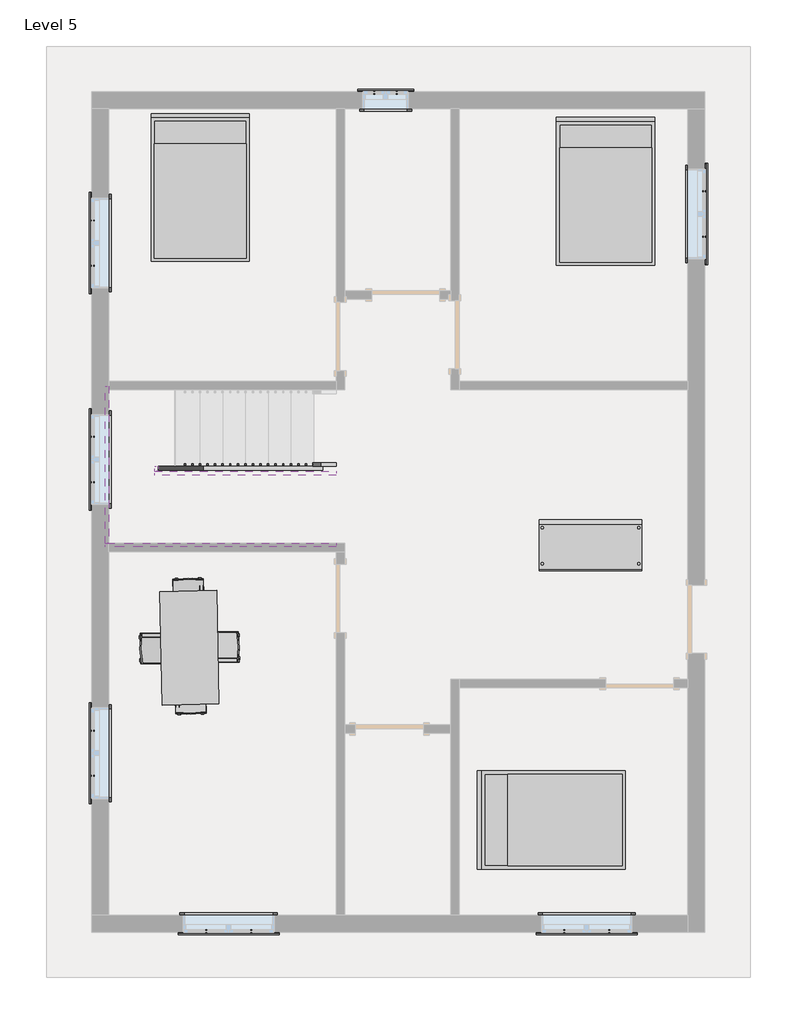
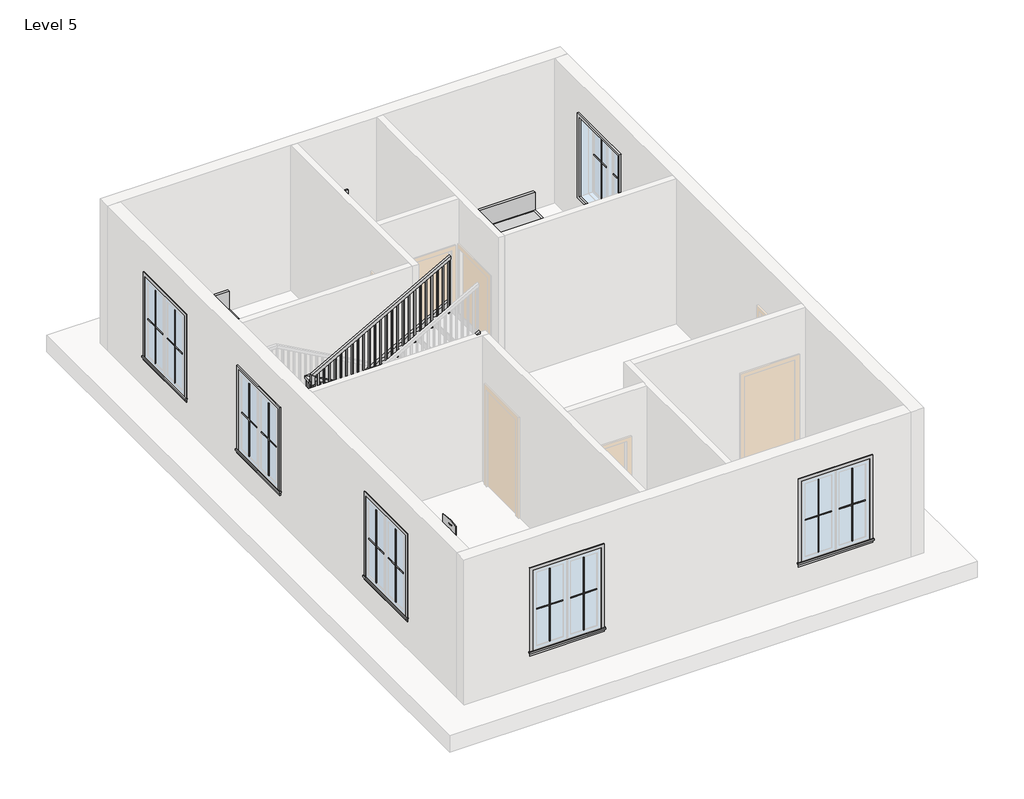
# One storey, part 2 of 2: 29 proxies, 6 members, 4 furniture elements, 1 railing.
"""IFC4 building model written with IfcOpenShell, lengths in millimetres."""

from ifc_helpers import new_model, si_unit, frame, origin, place, context, project, spatial, polyline, outline, extrude, faceted_brep, transform, mapped, element, save
from components import modern_coffee_table_17989_modern_coffee_table_17989_d3a860c8, muntin_pattern_2x2_muntin_pattern_2x2_6dad3731, muntin_pattern_2x2_muntin_pattern_2x2_a30a3345, muntin_pattern_2x2_muntin_pattern_2x2_53152e2c, muntin_pattern_2x2_muntin_pattern_2x2_e8f3e573, trim_window_exterior_flat_with_sill_92b9b949, trim_window_exterior_flat_with_sill_a665a915, trim_window_interior_flat_picture_frame_3bb882cf, trim_window_interior_flat_picture_frame_d485c387, bed_17739_bed_17739_15c61121, dining_table_w_chairs_11374_0cdfc61b

model = new_model("IFC4")

# Units and contexts
model_context = context("Model", 3, world=origin())
ifc_project = project(units=[si_unit("LENGTHUNIT", "METRE", prefix="MILLI")], contexts=[model_context])

# Site, building, storey
site = spatial("IfcSite", under=ifc_project)
building = spatial("IfcBuilding", under=site)
storey = spatial("IfcBuildingStorey", under=building, Name="Level 5", Elevation=12192.0)

# Proxies
placement = place(None, origin())
modern_coffee_table_17989_modern_coffee_table_17989_shape = modern_coffee_table_17989_modern_coffee_table_17989_d3a860c8(model_context)
element("IfcBuildingElementProxy", 1, Name="Modern_Coffee_Table_17989 : Modern_Coffee_Table_17989", ObjectType="Modern_Coffee_Table_17989 : Modern_Coffee_Table_17989", at=placement, inside=storey, context=model_context, shape_type="MappedRepresentation", body=[
    mapped(modern_coffee_table_17989_modern_coffee_table_17989_shape, transform((7937.5, 8234.1992646, 12192.0), x_axis=(1.0, 0.0, 0.0), y_axis=(0.0, 1.0, 0.0), z_axis=(0.0, 0.0, 1.0))),
])
muntin_pattern_2x2_muntin_pattern_2x2_shape = muntin_pattern_2x2_muntin_pattern_2x2_6dad3731(model_context)
element("IfcBuildingElementProxy", 2, Name="Muntin Pattern_2x2 : Muntin Pattern_2x2", ObjectType="Muntin Pattern_2x2 : Muntin Pattern_2x2", at=placement, inside=storey, context=model_context, shape_type="MappedRepresentation", body=[
    mapped(muntin_pattern_2x2_muntin_pattern_2x2_shape, transform((7961.3125, 2701.925, 13176.25), x_axis=(-1.0, 0.0, 0.0), y_axis=(0.0, -1.0, 0.0), z_axis=(0.0, 0.0, 1.0))),
])
element("IfcBuildingElementProxy", 3, Name="Muntin Pattern_2x2 : Muntin Pattern_2x2", ObjectType="Muntin Pattern_2x2 : Muntin Pattern_2x2", at=placement, inside=storey, context=model_context, shape_type="MappedRepresentation", body=[
    mapped(muntin_pattern_2x2_muntin_pattern_2x2_shape, transform((3154.3625, 2701.925, 13176.25), x_axis=(-1.0, 0.0, 0.0), y_axis=(0.0, -1.0, 0.0), z_axis=(0.0, 0.0, 1.0))),
])
element("IfcBuildingElementProxy", 4, Name="Muntin Pattern_2x2 : Muntin Pattern_2x2", ObjectType="Muntin Pattern_2x2 : Muntin Pattern_2x2", at=placement, inside=storey, context=model_context, shape_type="MappedRepresentation", body=[
    mapped(muntin_pattern_2x2_muntin_pattern_2x2_shape, transform((1025.525, 4789.4875, 13176.25), x_axis=(0.0, 1.0, 0.0), y_axis=(-1.0, 0.0, 0.0), z_axis=(0.0, 0.0, 1.0))),
])
element("IfcBuildingElementProxy", 5, Name="Muntin Pattern_2x2 : Muntin Pattern_2x2", ObjectType="Muntin Pattern_2x2 : Muntin Pattern_2x2", at=placement, inside=storey, context=model_context, shape_type="MappedRepresentation", body=[
    mapped(muntin_pattern_2x2_muntin_pattern_2x2_shape, transform((1025.525, 8732.8375, 13176.25), x_axis=(0.0, 1.0, 0.0), y_axis=(-1.0, 0.0, 0.0), z_axis=(0.0, 0.0, 1.0))),
])
element("IfcBuildingElementProxy", 6, Name="Muntin Pattern_2x2 : Muntin Pattern_2x2", ObjectType="Muntin Pattern_2x2 : Muntin Pattern_2x2", at=placement, inside=storey, context=model_context, shape_type="MappedRepresentation", body=[
    mapped(muntin_pattern_2x2_muntin_pattern_2x2_shape, transform((1025.525, 11637.9625, 13176.25), x_axis=(0.0, 1.0, 0.0), y_axis=(-1.0, 0.0, 0.0), z_axis=(0.0, 0.0, 1.0))),
])
element("IfcBuildingElementProxy", 7, Name="Muntin Pattern_2x2 : Muntin Pattern_2x2", ObjectType="Muntin Pattern_2x2 : Muntin Pattern_2x2", at=placement, inside=storey, context=model_context, shape_type="MappedRepresentation", body=[
    mapped(muntin_pattern_2x2_muntin_pattern_2x2_shape, transform((9236.075, 12634.9125, 13176.25), x_axis=(0.0, -1.0, 0.0), y_axis=(1.0, 0.0, 0.0), z_axis=(0.0, 0.0, 1.0))),
])
muntin_pattern_2x2_muntin_pattern_2x2_2_shape = muntin_pattern_2x2_muntin_pattern_2x2_a30a3345(model_context)
element("IfcBuildingElementProxy", 8, Name="Muntin Pattern_2x2 : Muntin Pattern_2x2", ObjectType="Muntin Pattern_2x2 : Muntin Pattern_2x2", at=placement, inside=storey, context=model_context, shape_type="MappedRepresentation", body=[
    mapped(muntin_pattern_2x2_muntin_pattern_2x2_2_shape, transform((7354.8875, 2701.925, 13176.25), x_axis=(1.0, 0.0, 0.0), y_axis=(0.0, 1.0, 0.0), z_axis=(0.0, 0.0, 1.0))),
])
element("IfcBuildingElementProxy", 9, Name="Muntin Pattern_2x2 : Muntin Pattern_2x2", ObjectType="Muntin Pattern_2x2 : Muntin Pattern_2x2", at=placement, inside=storey, context=model_context, shape_type="MappedRepresentation", body=[
    mapped(muntin_pattern_2x2_muntin_pattern_2x2_2_shape, transform((2547.9375, 2701.925, 13176.25), x_axis=(1.0, 0.0, 0.0), y_axis=(0.0, 1.0, 0.0), z_axis=(0.0, 0.0, 1.0))),
])
element("IfcBuildingElementProxy", 10, Name="Muntin Pattern_2x2 : Muntin Pattern_2x2", ObjectType="Muntin Pattern_2x2 : Muntin Pattern_2x2", at=placement, inside=storey, context=model_context, shape_type="MappedRepresentation", body=[
    mapped(muntin_pattern_2x2_muntin_pattern_2x2_2_shape, transform((1025.525, 5395.9125, 13176.25), x_axis=(0.0, -1.0, 0.0), y_axis=(1.0, 0.0, 0.0), z_axis=(0.0, 0.0, 1.0))),
])
element("IfcBuildingElementProxy", 11, Name="Muntin Pattern_2x2 : Muntin Pattern_2x2", ObjectType="Muntin Pattern_2x2 : Muntin Pattern_2x2", at=placement, inside=storey, context=model_context, shape_type="MappedRepresentation", body=[
    mapped(muntin_pattern_2x2_muntin_pattern_2x2_2_shape, transform((1025.525, 9339.2625, 13176.25), x_axis=(0.0, -1.0, 0.0), y_axis=(1.0, 0.0, 0.0), z_axis=(0.0, 0.0, 1.0))),
])
element("IfcBuildingElementProxy", 12, Name="Muntin Pattern_2x2 : Muntin Pattern_2x2", ObjectType="Muntin Pattern_2x2 : Muntin Pattern_2x2", at=placement, inside=storey, context=model_context, shape_type="MappedRepresentation", body=[
    mapped(muntin_pattern_2x2_muntin_pattern_2x2_2_shape, transform((1025.525, 12244.3875, 13176.25), x_axis=(0.0, -1.0, 0.0), y_axis=(1.0, 0.0, 0.0), z_axis=(0.0, 0.0, 1.0))),
])
element("IfcBuildingElementProxy", 13, Name="Muntin Pattern_2x2 : Muntin Pattern_2x2", ObjectType="Muntin Pattern_2x2 : Muntin Pattern_2x2", at=placement, inside=storey, context=model_context, shape_type="MappedRepresentation", body=[
    mapped(muntin_pattern_2x2_muntin_pattern_2x2_2_shape, transform((9236.075, 12028.4875, 13176.25), x_axis=(0.0, 1.0, 0.0), y_axis=(-1.0, 0.0, 0.0), z_axis=(0.0, 0.0, 1.0))),
])
muntin_pattern_2x2_muntin_pattern_2x2_3_shape = muntin_pattern_2x2_muntin_pattern_2x2_53152e2c(model_context)
element("IfcBuildingElementProxy", 14, Name="Muntin Pattern_2x2 : Muntin Pattern_2x2", ObjectType="Muntin Pattern_2x2 : Muntin Pattern_2x2", at=placement, inside=storey, context=model_context, shape_type="MappedRepresentation", body=[
    mapped(muntin_pattern_2x2_muntin_pattern_2x2_3_shape, transform((4808.5375, 13960.475, 13176.25), x_axis=(1.0, 0.0, 0.0), y_axis=(0.0, 1.0, 0.0), z_axis=(0.0, 0.0, 1.0))),
])
muntin_pattern_2x2_muntin_pattern_2x2_4_shape = muntin_pattern_2x2_muntin_pattern_2x2_e8f3e573(model_context)
element("IfcBuildingElementProxy", 15, Name="Muntin Pattern_2x2 : Muntin Pattern_2x2", ObjectType="Muntin Pattern_2x2 : Muntin Pattern_2x2", at=placement, inside=storey, context=model_context, shape_type="MappedRepresentation", body=[
    mapped(muntin_pattern_2x2_muntin_pattern_2x2_4_shape, transform((5110.1625, 13960.475, 13176.25), x_axis=(-1.0, 0.0, 0.0), y_axis=(0.0, -1.0, 0.0), z_axis=(0.0, 0.0, 1.0))),
])
trim_window_exterior_flat_with_sill_shape = trim_window_exterior_flat_with_sill_92b9b949(model_context)
element("IfcBuildingElementProxy", 16, Name="Trim-Window-Exterior-Flat : with Sill", ObjectType="Trim-Window-Exterior-Flat : with Sill", at=placement, inside=storey, context=model_context, shape_type="MappedRepresentation", body=[
    mapped(trim_window_exterior_flat_with_sill_shape, transform((7658.1, 2692.4, 14630.4), x_axis=(1.0, 0.0, 0.0), y_axis=(0.0, 0.0, 1.0), z_axis=(0.0, -1.0, 0.0))),
])
element("IfcBuildingElementProxy", 17, Name="Trim-Window-Exterior-Flat : with Sill", ObjectType="Trim-Window-Exterior-Flat : with Sill", at=placement, inside=storey, context=model_context, shape_type="MappedRepresentation", body=[
    mapped(trim_window_exterior_flat_with_sill_shape, transform((2851.15, 2692.4, 14630.4), x_axis=(1.0, 0.0, 0.0), y_axis=(0.0, 0.0, 1.0), z_axis=(0.0, -1.0, 0.0))),
])
element("IfcBuildingElementProxy", 18, Name="Trim-Window-Exterior-Flat : with Sill", ObjectType="Trim-Window-Exterior-Flat : with Sill", at=placement, inside=storey, context=model_context, shape_type="MappedRepresentation", body=[
    mapped(trim_window_exterior_flat_with_sill_shape, transform((1016.0, 5092.7, 14630.4), x_axis=(0.0, -1.0, 0.0), y_axis=(0.0, 0.0, 1.0), z_axis=(-1.0, 0.0, 0.0))),
])
element("IfcBuildingElementProxy", 19, Name="Trim-Window-Exterior-Flat : with Sill", ObjectType="Trim-Window-Exterior-Flat : with Sill", at=placement, inside=storey, context=model_context, shape_type="MappedRepresentation", body=[
    mapped(trim_window_exterior_flat_with_sill_shape, transform((1016.0, 9036.05, 14630.4), x_axis=(0.0, -1.0, 0.0), y_axis=(0.0, 0.0, 1.0), z_axis=(-1.0, 0.0, 0.0))),
])
element("IfcBuildingElementProxy", 20, Name="Trim-Window-Exterior-Flat : with Sill", ObjectType="Trim-Window-Exterior-Flat : with Sill", at=placement, inside=storey, context=model_context, shape_type="MappedRepresentation", body=[
    mapped(trim_window_exterior_flat_with_sill_shape, transform((1016.0, 11941.175, 14630.4), x_axis=(0.0, -1.0, 0.0), y_axis=(0.0, 0.0, 1.0), z_axis=(-1.0, 0.0, 0.0))),
])
element("IfcBuildingElementProxy", 21, Name="Trim-Window-Exterior-Flat : with Sill", ObjectType="Trim-Window-Exterior-Flat : with Sill", at=placement, inside=storey, context=model_context, shape_type="MappedRepresentation", body=[
    mapped(trim_window_exterior_flat_with_sill_shape, transform((9245.6, 12331.7, 14630.4), x_axis=(0.0, 1.0, 0.0), y_axis=(0.0, 0.0, 1.0), z_axis=(1.0, 0.0, 0.0))),
])
trim_window_exterior_flat_with_sill_2_shape = trim_window_exterior_flat_with_sill_a665a915(model_context)
element("IfcBuildingElementProxy", 22, Name="Trim-Window-Exterior-Flat : with Sill", ObjectType="Trim-Window-Exterior-Flat : with Sill", at=placement, inside=storey, context=model_context, shape_type="MappedRepresentation", body=[
    mapped(trim_window_exterior_flat_with_sill_2_shape, transform((4959.35, 13970.0, 14020.8), x_axis=(-1.0, 0.0, 0.0), y_axis=(0.0, 0.0, 1.0), z_axis=(0.0, 1.0, 0.0))),
])
trim_window_interior_flat_picture_frame_shape = trim_window_interior_flat_picture_frame_3bb882cf(model_context)
element("IfcBuildingElementProxy", 23, Name="Trim-Window-Interior-Flat : Picture Frame", ObjectType="Trim-Window-Interior-Flat : Picture Frame", at=placement, inside=storey, context=model_context, shape_type="MappedRepresentation", body=[
    mapped(trim_window_interior_flat_picture_frame_shape, transform((7658.1, 2921.0, 14630.4), x_axis=(-1.0, 0.0, 0.0), y_axis=(0.0, 0.0, 1.0), z_axis=(0.0, 1.0, 0.0))),
])
element("IfcBuildingElementProxy", 24, Name="Trim-Window-Interior-Flat : Picture Frame", ObjectType="Trim-Window-Interior-Flat : Picture Frame", at=placement, inside=storey, context=model_context, shape_type="MappedRepresentation", body=[
    mapped(trim_window_interior_flat_picture_frame_shape, transform((2851.15, 2921.0, 14630.4), x_axis=(-1.0, 0.0, 0.0), y_axis=(0.0, 0.0, 1.0), z_axis=(0.0, 1.0, 0.0))),
])
element("IfcBuildingElementProxy", 25, Name="Trim-Window-Interior-Flat : Picture Frame", ObjectType="Trim-Window-Interior-Flat : Picture Frame", at=placement, inside=storey, context=model_context, shape_type="MappedRepresentation", body=[
    mapped(trim_window_interior_flat_picture_frame_shape, transform((1244.6, 5092.7, 14630.4), x_axis=(0.0, 1.0, 0.0), y_axis=(0.0, 0.0, 1.0), z_axis=(1.0, 0.0, 0.0))),
])
element("IfcBuildingElementProxy", 26, Name="Trim-Window-Interior-Flat : Picture Frame", ObjectType="Trim-Window-Interior-Flat : Picture Frame", at=placement, inside=storey, context=model_context, shape_type="MappedRepresentation", body=[
    mapped(trim_window_interior_flat_picture_frame_shape, transform((1244.6, 9036.05, 14630.4), x_axis=(0.0, 1.0, 0.0), y_axis=(0.0, 0.0, 1.0), z_axis=(1.0, 0.0, 0.0))),
])
element("IfcBuildingElementProxy", 27, Name="Trim-Window-Interior-Flat : Picture Frame", ObjectType="Trim-Window-Interior-Flat : Picture Frame", at=placement, inside=storey, context=model_context, shape_type="MappedRepresentation", body=[
    mapped(trim_window_interior_flat_picture_frame_shape, transform((1244.6, 11941.175, 14630.4), x_axis=(0.0, 1.0, 0.0), y_axis=(0.0, 0.0, 1.0), z_axis=(1.0, 0.0, 0.0))),
])
element("IfcBuildingElementProxy", 28, Name="Trim-Window-Interior-Flat : Picture Frame", ObjectType="Trim-Window-Interior-Flat : Picture Frame", at=placement, inside=storey, context=model_context, shape_type="MappedRepresentation", body=[
    mapped(trim_window_interior_flat_picture_frame_shape, transform((9017.0, 12331.7, 14630.4), x_axis=(0.0, -1.0, 0.0), y_axis=(0.0, 0.0, 1.0), z_axis=(-1.0, 0.0, 0.0))),
])
trim_window_interior_flat_picture_frame_2_shape = trim_window_interior_flat_picture_frame_d485c387(model_context)
element("IfcBuildingElementProxy", 29, Name="Trim-Window-Interior-Flat : Picture Frame", ObjectType="Trim-Window-Interior-Flat : Picture Frame", at=placement, inside=storey, context=model_context, shape_type="MappedRepresentation", body=[
    mapped(trim_window_interior_flat_picture_frame_2_shape, transform((4959.35, 13741.4, 14020.8), x_axis=(1.0, 0.0, 0.0), y_axis=(0.0, 0.0, 1.0), z_axis=(0.0, -1.0, 0.0))),
])

# Furniture
bed_17739_bed_17739_shape = bed_17739_bed_17739_15c61121(model_context)
element("IfcFurniture", 30, ObjectType="Bed_17739 : Bed_17739", at=placement, inside=storey, context=model_context, shape_type="MappedRepresentation", body=[
    mapped(bed_17739_bed_17739_shape, transform((2470.15, 12661.9, 12192.0), x_axis=(1.0, 0.0, 0.0), y_axis=(0.0, 1.0, 0.0), z_axis=(0.0, 0.0, 1.0))),
])
element("IfcFurniture", 31, ObjectType="Bed_17739 : Bed_17739", at=placement, inside=storey, context=model_context, shape_type="MappedRepresentation", body=[
    mapped(bed_17739_bed_17739_shape, transform((7912.1, 12611.1, 12192.0), x_axis=(1.0, 0.0, 0.0), y_axis=(0.0, 1.0, 0.0), z_axis=(0.0, 0.0, 1.0))),
])
element("IfcFurniture", 32, ObjectType="Bed_17739 : Bed_17739", at=placement, inside=storey, context=model_context, shape_type="MappedRepresentation", body=[
    mapped(bed_17739_bed_17739_shape, transform((7207.25, 4197.35, 12192.0), x_axis=(0.0, 1.0, 0.0), y_axis=(-1.0, 0.0, 0.0), z_axis=(0.0, 0.0, 1.0))),
])
dining_table_w_chairs_11374_shape = dining_table_w_chairs_11374_0cdfc61b(model_context)
element("IfcFurniture", 33, ObjectType="Dining_Table_w_Chairs_11374", at=placement, inside=storey, context=model_context, shape_type="MappedRepresentation", body=[
    mapped(dining_table_w_chairs_11374_shape, transform((2420.6366388, 6492.5326572, 12192.0), x_axis=(-0.019560245774115807, 0.9998086800909743, 0.0), y_axis=(-0.9998086800909743, -0.019560245774115807, 0.0), z_axis=(0.0, 0.0, 1.0))),
])

# Members
element("IfcMember", 34, ObjectType="Stringer - 2\" Width", at=placement, inside=storey, context=model_context, shape_type="SweptSolid", body=[
    extrude(outline(polyline([(12192.0, 4295.1355783), (12399.5983948, 4295.1355783), (13726.0428392, 1907.5355783), (13377.3641651, 1907.5355783), (12192.0, 4041.1910755), (12192.0, 4295.1355783)])), frame((0.0, 8893.8068332, 0.0), z_axis=(0.0, 1.0, 0.0), x_axis=(0.0, 0.0, 1.0)), (0.0, 0.0, 1.0), 50.8),
])
element("IfcMember", 35, ObjectType="Stringer - 2\" Width", at=placement, inside=storey, context=model_context, shape_type="SweptSolid", body=[
    extrude(outline(polyline([(1856.7355783, 8944.6068332), (1907.5355783, 8944.6068332), (1907.5355783, 8877.3), (1856.7355783, 8877.3), (1856.7355783, 8944.6068332)])), frame((0.0, 0.0, 13487.4), z_axis=(0.0, 0.0, 1.0), x_axis=(1.0, 0.0, 0.0)), (0.0, 0.0, 1.0), 304.8),
])
element("IfcMember", 36, ObjectType="Stringer - 2\" Width", at=placement, inside=storey, context=model_context, shape_type="SweptSolid", body=[
    extrude(outline(polyline([(13923.5983948, 1856.7355783), (13574.9197207, 1856.7355783), (14929.5863873, 4295.1355783), (15278.2650614, 4295.1355783), (13923.5983948, 1856.7355783)])), frame((0.0, 8826.5, 0.0), z_axis=(0.0, 1.0, 0.0), x_axis=(0.0, 0.0, 1.0)), (0.0, 0.0, 1.0), 50.8),
])
element("IfcMember", 37, ObjectType="Stringer - 2\" Width", at=placement, inside=storey, context=model_context, shape_type="SweptSolid", body=[
    extrude(outline(polyline([(12192.0, 4295.1355783), (12399.5983948, 4295.1355783), (13792.2, 1788.4526889), (13792.2, 1244.6), (13745.6617086, 1244.6), (12192.0, 4041.1910755), (12192.0, 4295.1355783)])), frame((0.0, 9969.5, 0.0), z_axis=(0.0, 1.0, 0.0), x_axis=(0.0, 0.0, 1.0)), (0.0, 0.0, 1.0), 50.8),
])
element("IfcMember", 38, ObjectType="Stringer - 2\" Width", at=placement, inside=storey, context=model_context, shape_type="SweptSolid", body=[
    extrude(outline(polyline([(1193.8, 10020.3), (1244.6, 10020.3), (1244.6, 7912.1), (1193.8, 7912.1), (1193.8, 10020.3)])), frame((0.0, 0.0, 13487.4), z_axis=(0.0, 0.0, 1.0), x_axis=(1.0, 0.0, 0.0)), (0.0, 0.0, 1.0), 304.8),
])
element("IfcMember", 39, ObjectType="Stringer - 2\" Width", at=placement, inside=storey, context=model_context, shape_type="SweptSolid", body=[
    extrude(outline(polyline([(13555.3008513, 1193.8), (13487.4, 1193.8), (13487.4, 1699.2000811), (14929.5863873, 4295.1355783), (15278.2650614, 4295.1355783), (13555.3008513, 1193.8)])), frame((0.0, 7861.3, 0.0), z_axis=(0.0, 1.0, 0.0), x_axis=(0.0, 0.0, 1.0)), (0.0, 0.0, 1.0), 50.8),
])

# Railing
element("IfcRailing", 40, ObjectType="Handrail - Rectangular", at=placement, inside=storey, context=model_context, shape_type="SolidModel", body=[
    faceted_brep([(4295.1355783, 8944.6068332, 13275.7333333), (4295.1355783, 8944.6068332, 13217.620221), (4295.1355783, 8995.4068332, 13217.620221), (4295.1355783, 8995.4068332, 13275.7333333), (1932.9355783, 8944.6068332, 14588.0666667), (1882.1355783, 8944.6068332, 14558.1757765), (1882.1355783, 8995.4068332, 14558.1757765), (1932.9355783, 8995.4068332, 14588.0666667), (1932.9355783, 8944.6068332, 14630.4), (1882.1355783, 8944.6068332, 14579.6), (1882.1355783, 8995.4068332, 14579.6), (1932.9355783, 8995.4068332, 14630.4), (1856.7355783, 8944.6068332, 14630.4), (1856.7355783, 8944.6068332, 14579.6), (1805.9355783, 8995.4068332, 14579.6), (1805.9355783, 8995.4068332, 14630.4), (1856.7355783, 8868.4068332, 14630.4), (1856.7355783, 8868.4068332, 14579.6), (1805.9355783, 8868.4068332, 14579.6), (1805.9355783, 8868.4068332, 14630.4), (1856.7355783, 8826.5, 14630.4), (1805.9355783, 8826.5, 14630.4), (1805.9355783, 8775.7, 14579.6), (1856.7355783, 8775.7, 14579.6)], [[[0, 1, 2, 3]], [[1, 0, 4, 5]], [[2, 1, 5, 6]], [[3, 2, 6, 7]], [[0, 3, 7, 4]], [[5, 4, 8, 9]], [[6, 5, 9, 10]], [[7, 6, 10, 11]], [[4, 7, 11, 8]], [[9, 8, 12, 13]], [[10, 9, 13, 14]], [[11, 10, 14, 15]], [[8, 11, 15, 12]], [[13, 12, 16, 17]], [[14, 13, 17, 18]], [[15, 14, 18, 19]], [[12, 15, 19, 16]], [[20, 21, 22, 23]], [[17, 16, 20, 23]], [[18, 17, 23, 22]], [[19, 18, 22, 21]], [[16, 19, 21, 20]]]),
    faceted_brep([(1856.7355783, 8826.5, 14630.4), (1856.7355783, 8775.7, 14579.6), (1805.9355783, 8775.7, 14579.6), (1805.9355783, 8826.5, 14630.4), (1856.7355783, 8826.5, 14741.620221), (1805.9355783, 8826.5, 14771.5111111), (1805.9355783, 8775.7, 14771.5111111), (1856.7355783, 8775.7, 14741.620221)], [[[0, 1, 2, 3]], [[4, 5, 6, 7]], [[1, 0, 4, 7]], [[2, 1, 7, 6]], [[3, 2, 6, 5]], [[0, 3, 5, 4]]]),
    faceted_brep([(1805.9355783, 8826.5, 14771.5111111), (1856.7355783, 8826.5, 14741.620221), (1856.7355783, 8775.7, 14741.620221), (1805.9355783, 8775.7, 14771.5111111), (4295.1355783, 8826.5, 16154.4), (4295.1355783, 8775.7, 16154.4), (4295.1355783, 8775.7, 16096.2868876), (4295.1355783, 8826.5, 16096.2868876)], [[[0, 1, 2, 3]], [[4, 5, 6, 7]], [[1, 0, 4, 7]], [[2, 1, 7, 6]], [[3, 2, 6, 5]], [[0, 3, 5, 4]]]),
    extrude(outline(polyline([(16076.8841099, 4260.2105783), (15070.6666667, 4260.2105783), (15070.6666667, 4279.2605783), (16087.4674432, 4279.2605783), (16076.8841099, 4260.2105783)])), frame((0.0, 8791.575, 0.0), z_axis=(0.0, 1.0, 0.0), x_axis=(0.0, 0.0, 1.0)), (0.0, 0.0, 1.0), 19.05),
    extrude(outline(polyline([(16020.4396654, 4158.6105783), (15070.6666667, 4158.6105783), (15070.6666667, 4177.6605783), (16031.0229988, 4177.6605783), (16020.4396654, 4158.6105783)])), frame((0.0, 8791.575, 0.0), z_axis=(0.0, 1.0, 0.0), x_axis=(0.0, 0.0, 1.0)), (0.0, 0.0, 1.0), 19.05),
    extrude(outline(polyline([(15963.995221, 4057.0105783), (15070.6666667, 4057.0105783), (15070.6666667, 4076.0605783), (15974.5785543, 4076.0605783), (15963.995221, 4057.0105783)])), frame((0.0, 8791.575, 0.0), z_axis=(0.0, 1.0, 0.0), x_axis=(0.0, 0.0, 1.0)), (0.0, 0.0, 1.0), 19.05),
    extrude(outline(polyline([(15907.5507765, 3955.4105783), (14901.3333333, 3955.4105783), (14901.3333333, 3974.4605783), (15918.1341099, 3974.4605783), (15907.5507765, 3955.4105783)])), frame((0.0, 8791.575, 0.0), z_axis=(0.0, 1.0, 0.0), x_axis=(0.0, 0.0, 1.0)), (0.0, 0.0, 1.0), 19.05),
    extrude(outline(polyline([(15851.1063321, 3853.8105783), (14901.3333333, 3853.8105783), (14901.3333333, 3872.8605783), (15861.6896654, 3872.8605783), (15851.1063321, 3853.8105783)])), frame((0.0, 8791.575, 0.0), z_axis=(0.0, 1.0, 0.0), x_axis=(0.0, 0.0, 1.0)), (0.0, 0.0, 1.0), 19.05),
    extrude(outline(polyline([(15794.6618876, 3752.2105783), (14901.3333333, 3752.2105783), (14901.3333333, 3771.2605783), (15805.245221, 3771.2605783), (15794.6618876, 3752.2105783)])), frame((0.0, 8791.575, 0.0), z_axis=(0.0, 1.0, 0.0), x_axis=(0.0, 0.0, 1.0)), (0.0, 0.0, 1.0), 19.05),
    extrude(outline(polyline([(15738.2174432, 3650.6105783), (14732.0, 3650.6105783), (14732.0, 3669.6605783), (15748.8007765, 3669.6605783), (15738.2174432, 3650.6105783)])), frame((0.0, 8791.575, 0.0), z_axis=(0.0, 1.0, 0.0), x_axis=(0.0, 0.0, 1.0)), (0.0, 0.0, 1.0), 19.05),
    extrude(outline(polyline([(15681.7729988, 3549.0105783), (14732.0, 3549.0105783), (14732.0, 3568.0605783), (15692.3563321, 3568.0605783), (15681.7729988, 3549.0105783)])), frame((0.0, 8791.575, 0.0), z_axis=(0.0, 1.0, 0.0), x_axis=(0.0, 0.0, 1.0)), (0.0, 0.0, 1.0), 19.05),
    extrude(outline(polyline([(15625.3285543, 3447.4105783), (14732.0, 3447.4105783), (14732.0, 3466.4605783), (15635.9118876, 3466.4605783), (15625.3285543, 3447.4105783)])), frame((0.0, 8791.575, 0.0), z_axis=(0.0, 1.0, 0.0), x_axis=(0.0, 0.0, 1.0)), (0.0, 0.0, 1.0), 19.05),
    extrude(outline(polyline([(15568.8841099, 3345.8105783), (14562.6666667, 3345.8105783), (14562.6666667, 3364.8605783), (15579.4674432, 3364.8605783), (15568.8841099, 3345.8105783)])), frame((0.0, 8791.575, 0.0), z_axis=(0.0, 1.0, 0.0), x_axis=(0.0, 0.0, 1.0)), (0.0, 0.0, 1.0), 19.05),
    extrude(outline(polyline([(15512.4396654, 3244.2105783), (14562.6666667, 3244.2105783), (14562.6666667, 3263.2605783), (15523.0229988, 3263.2605783), (15512.4396654, 3244.2105783)])), frame((0.0, 8791.575, 0.0), z_axis=(0.0, 1.0, 0.0), x_axis=(0.0, 0.0, 1.0)), (0.0, 0.0, 1.0), 19.05),
    extrude(outline(polyline([(15455.995221, 3142.6105783), (14562.6666667, 3142.6105783), (14562.6666667, 3161.6605783), (15466.5785543, 3161.6605783), (15455.995221, 3142.6105783)])), frame((0.0, 8791.575, 0.0), z_axis=(0.0, 1.0, 0.0), x_axis=(0.0, 0.0, 1.0)), (0.0, 0.0, 1.0), 19.05),
    extrude(outline(polyline([(15399.5507765, 3041.0105783), (14393.3333333, 3041.0105783), (14393.3333333, 3060.0605783), (15410.1341099, 3060.0605783), (15399.5507765, 3041.0105783)])), frame((0.0, 8791.575, 0.0), z_axis=(0.0, 1.0, 0.0), x_axis=(0.0, 0.0, 1.0)), (0.0, 0.0, 1.0), 19.05),
    extrude(outline(polyline([(15343.1063321, 2939.4105783), (14393.3333333, 2939.4105783), (14393.3333333, 2958.4605783), (15353.6896654, 2958.4605783), (15343.1063321, 2939.4105783)])), frame((0.0, 8791.575, 0.0), z_axis=(0.0, 1.0, 0.0), x_axis=(0.0, 0.0, 1.0)), (0.0, 0.0, 1.0), 19.05),
    extrude(outline(polyline([(15286.6618876, 2837.8105783), (14393.3333333, 2837.8105783), (14393.3333333, 2856.8605783), (15297.245221, 2856.8605783), (15286.6618876, 2837.8105783)])), frame((0.0, 8791.575, 0.0), z_axis=(0.0, 1.0, 0.0), x_axis=(0.0, 0.0, 1.0)), (0.0, 0.0, 1.0), 19.05),
    extrude(outline(polyline([(15230.2174432, 2736.2105783), (14224.0, 2736.2105783), (14224.0, 2755.2605783), (15240.8007765, 2755.2605783), (15230.2174432, 2736.2105783)])), frame((0.0, 8791.575, 0.0), z_axis=(0.0, 1.0, 0.0), x_axis=(0.0, 0.0, 1.0)), (0.0, 0.0, 1.0), 19.05),
    extrude(outline(polyline([(15173.7729988, 2634.6105783), (14224.0, 2634.6105783), (14224.0, 2653.6605783), (15184.3563321, 2653.6605783), (15173.7729988, 2634.6105783)])), frame((0.0, 8791.575, 0.0), z_axis=(0.0, 1.0, 0.0), x_axis=(0.0, 0.0, 1.0)), (0.0, 0.0, 1.0), 19.05),
    extrude(outline(polyline([(15117.3285543, 2533.0105783), (14224.0, 2533.0105783), (14224.0, 2552.0605783), (15127.9118876, 2552.0605783), (15117.3285543, 2533.0105783)])), frame((0.0, 8791.575, 0.0), z_axis=(0.0, 1.0, 0.0), x_axis=(0.0, 0.0, 1.0)), (0.0, 0.0, 1.0), 19.05),
    extrude(outline(polyline([(15060.8841099, 2431.4105783), (14054.6666667, 2431.4105783), (14054.6666667, 2450.4605783), (15071.4674432, 2450.4605783), (15060.8841099, 2431.4105783)])), frame((0.0, 8791.575, 0.0), z_axis=(0.0, 1.0, 0.0), x_axis=(0.0, 0.0, 1.0)), (0.0, 0.0, 1.0), 19.05),
    extrude(outline(polyline([(15004.4396654, 2329.8105783), (14054.6666667, 2329.8105783), (14054.6666667, 2348.8605783), (15015.0229988, 2348.8605783), (15004.4396654, 2329.8105783)])), frame((0.0, 8791.575, 0.0), z_axis=(0.0, 1.0, 0.0), x_axis=(0.0, 0.0, 1.0)), (0.0, 0.0, 1.0), 19.05),
    extrude(outline(polyline([(14947.995221, 2228.2105783), (14054.6666667, 2228.2105783), (14054.6666667, 2247.2605783), (14958.5785543, 2247.2605783), (14947.995221, 2228.2105783)])), frame((0.0, 8791.575, 0.0), z_axis=(0.0, 1.0, 0.0), x_axis=(0.0, 0.0, 1.0)), (0.0, 0.0, 1.0), 19.05),
    extrude(outline(polyline([(14891.5507765, 2126.6105783), (13885.3333333, 2126.6105783), (13885.3333333, 2145.6605783), (14902.1341099, 2145.6605783), (14891.5507765, 2126.6105783)])), frame((0.0, 8791.575, 0.0), z_axis=(0.0, 1.0, 0.0), x_axis=(0.0, 0.0, 1.0)), (0.0, 0.0, 1.0), 19.05),
    extrude(outline(polyline([(14835.1063321, 2025.0105783), (13885.3333333, 2025.0105783), (13885.3333333, 2044.0605783), (14845.6896654, 2044.0605783), (14835.1063321, 2025.0105783)])), frame((0.0, 8791.575, 0.0), z_axis=(0.0, 1.0, 0.0), x_axis=(0.0, 0.0, 1.0)), (0.0, 0.0, 1.0), 19.05),
    extrude(outline(polyline([(14778.6618876, 1923.4105783), (13885.3333333, 1923.4105783), (13885.3333333, 1942.4605783), (14789.245221, 1942.4605783), (14778.6618876, 1923.4105783)])), frame((0.0, 8791.575, 0.0), z_axis=(0.0, 1.0, 0.0), x_axis=(0.0, 0.0, 1.0)), (0.0, 0.0, 1.0), 19.05),
    extrude(outline(polyline([(1840.8605783, 8877.9318332), (1840.8605783, 8858.8818332), (1821.8105783, 8858.8818332), (1821.8105783, 8877.9318332), (1840.8605783, 8877.9318332)])), frame((0.0, 0.0, 13716.0), z_axis=(0.0, 0.0, 1.0), x_axis=(1.0, 0.0, 0.0)), (0.0, 0.0, 1.0), 863.6),
    extrude(outline(polyline([(1866.2605783, 8960.4818332), (1847.2105783, 8960.4818332), (1847.2105783, 8979.5318332), (1866.2605783, 8979.5318332), (1866.2605783, 8960.4818332)])), frame((0.0, 0.0, 13716.0), z_axis=(0.0, 0.0, 1.0), x_axis=(1.0, 0.0, 0.0)), (0.0, 0.0, 1.0), 863.6),
    extrude(outline(polyline([(14521.1341099, 1948.8105783), (13546.6666667, 1948.8105783), (13546.6666667, 1967.8605783), (14510.5507765, 1967.8605783), (14521.1341099, 1948.8105783)])), frame((0.0, 8960.4818332, 0.0), z_axis=(0.0, 1.0, 0.0), x_axis=(0.0, 0.0, 1.0)), (0.0, 0.0, 1.0), 19.05),
    extrude(outline(polyline([(14464.6896654, 2050.4105783), (13546.6666667, 2050.4105783), (13546.6666667, 2069.4605783), (14454.1063321, 2069.4605783), (14464.6896654, 2050.4105783)])), frame((0.0, 8960.4818332, 0.0), z_axis=(0.0, 1.0, 0.0), x_axis=(0.0, 0.0, 1.0)), (0.0, 0.0, 1.0), 19.05),
    extrude(outline(polyline([(14408.245221, 2152.0105783), (13546.6666667, 2152.0105783), (13546.6666667, 2171.0605783), (14397.6618876, 2171.0605783), (14408.245221, 2152.0105783)])), frame((0.0, 8960.4818332, 0.0), z_axis=(0.0, 1.0, 0.0), x_axis=(0.0, 0.0, 1.0)), (0.0, 0.0, 1.0), 19.05),
    extrude(outline(polyline([(14351.8007765, 2253.6105783), (13377.3333333, 2253.6105783), (13377.3333333, 2272.6605783), (14341.2174432, 2272.6605783), (14351.8007765, 2253.6105783)])), frame((0.0, 8960.4818332, 0.0), z_axis=(0.0, 1.0, 0.0), x_axis=(0.0, 0.0, 1.0)), (0.0, 0.0, 1.0), 19.05),
    extrude(outline(polyline([(14295.3563321, 2355.2105783), (13377.3333333, 2355.2105783), (13377.3333333, 2374.2605783), (14284.7729988, 2374.2605783), (14295.3563321, 2355.2105783)])), frame((0.0, 8960.4818332, 0.0), z_axis=(0.0, 1.0, 0.0), x_axis=(0.0, 0.0, 1.0)), (0.0, 0.0, 1.0), 19.05),
    extrude(outline(polyline([(14238.9118876, 2456.8105783), (13377.3333333, 2456.8105783), (13377.3333333, 2475.8605783), (14228.3285543, 2475.8605783), (14238.9118876, 2456.8105783)])), frame((0.0, 8960.4818332, 0.0), z_axis=(0.0, 1.0, 0.0), x_axis=(0.0, 0.0, 1.0)), (0.0, 0.0, 1.0), 19.05),
    extrude(outline(polyline([(14182.4674432, 2558.4105783), (13208.0, 2558.4105783), (13208.0, 2577.4605783), (14171.8841099, 2577.4605783), (14182.4674432, 2558.4105783)])), frame((0.0, 8960.4818332, 0.0), z_axis=(0.0, 1.0, 0.0), x_axis=(0.0, 0.0, 1.0)), (0.0, 0.0, 1.0), 19.05),
    extrude(outline(polyline([(14126.0229988, 2660.0105783), (13208.0, 2660.0105783), (13208.0, 2679.0605783), (14115.4396654, 2679.0605783), (14126.0229988, 2660.0105783)])), frame((0.0, 8960.4818332, 0.0), z_axis=(0.0, 1.0, 0.0), x_axis=(0.0, 0.0, 1.0)), (0.0, 0.0, 1.0), 19.05),
    extrude(outline(polyline([(14069.5785543, 2761.6105783), (13208.0, 2761.6105783), (13208.0, 2780.6605783), (14058.995221, 2780.6605783), (14069.5785543, 2761.6105783)])), frame((0.0, 8960.4818332, 0.0), z_axis=(0.0, 1.0, 0.0), x_axis=(0.0, 0.0, 1.0)), (0.0, 0.0, 1.0), 19.05),
    extrude(outline(polyline([(14013.1341099, 2863.2105783), (13038.6666667, 2863.2105783), (13038.6666667, 2882.2605783), (14002.5507765, 2882.2605783), (14013.1341099, 2863.2105783)])), frame((0.0, 8960.4818332, 0.0), z_axis=(0.0, 1.0, 0.0), x_axis=(0.0, 0.0, 1.0)), (0.0, 0.0, 1.0), 19.05),
    extrude(outline(polyline([(13956.6896654, 2964.8105783), (13038.6666667, 2964.8105783), (13038.6666667, 2983.8605783), (13946.1063321, 2983.8605783), (13956.6896654, 2964.8105783)])), frame((0.0, 8960.4818332, 0.0), z_axis=(0.0, 1.0, 0.0), x_axis=(0.0, 0.0, 1.0)), (0.0, 0.0, 1.0), 19.05),
    extrude(outline(polyline([(13900.245221, 3066.4105783), (13038.6666667, 3066.4105783), (13038.6666667, 3085.4605783), (13889.6618876, 3085.4605783), (13900.245221, 3066.4105783)])), frame((0.0, 8960.4818332, 0.0), z_axis=(0.0, 1.0, 0.0), x_axis=(0.0, 0.0, 1.0)), (0.0, 0.0, 1.0), 19.05),
    extrude(outline(polyline([(13843.8007765, 3168.0105783), (12869.3333333, 3168.0105783), (12869.3333333, 3187.0605783), (13833.2174432, 3187.0605783), (13843.8007765, 3168.0105783)])), frame((0.0, 8960.4818332, 0.0), z_axis=(0.0, 1.0, 0.0), x_axis=(0.0, 0.0, 1.0)), (0.0, 0.0, 1.0), 19.05),
    extrude(outline(polyline([(13787.3563321, 3269.6105783), (12869.3333333, 3269.6105783), (12869.3333333, 3288.6605783), (13776.7729988, 3288.6605783), (13787.3563321, 3269.6105783)])), frame((0.0, 8960.4818332, 0.0), z_axis=(0.0, 1.0, 0.0), x_axis=(0.0, 0.0, 1.0)), (0.0, 0.0, 1.0), 19.05),
    extrude(outline(polyline([(13730.9118876, 3371.2105783), (12869.3333333, 3371.2105783), (12869.3333333, 3390.2605783), (13720.3285543, 3390.2605783), (13730.9118876, 3371.2105783)])), frame((0.0, 8960.4818332, 0.0), z_axis=(0.0, 1.0, 0.0), x_axis=(0.0, 0.0, 1.0)), (0.0, 0.0, 1.0), 19.05),
    extrude(outline(polyline([(13674.4674432, 3472.8105783), (12700.0, 3472.8105783), (12700.0, 3491.8605783), (13663.8841099, 3491.8605783), (13674.4674432, 3472.8105783)])), frame((0.0, 8960.4818332, 0.0), z_axis=(0.0, 1.0, 0.0), x_axis=(0.0, 0.0, 1.0)), (0.0, 0.0, 1.0), 19.05),
    extrude(outline(polyline([(13618.0229988, 3574.4105783), (12700.0, 3574.4105783), (12700.0, 3593.4605783), (13607.4396654, 3593.4605783), (13618.0229988, 3574.4105783)])), frame((0.0, 8960.4818332, 0.0), z_axis=(0.0, 1.0, 0.0), x_axis=(0.0, 0.0, 1.0)), (0.0, 0.0, 1.0), 19.05),
    extrude(outline(polyline([(13561.5785543, 3676.0105783), (12700.0, 3676.0105783), (12700.0, 3695.0605783), (13550.995221, 3695.0605783), (13561.5785543, 3676.0105783)])), frame((0.0, 8960.4818332, 0.0), z_axis=(0.0, 1.0, 0.0), x_axis=(0.0, 0.0, 1.0)), (0.0, 0.0, 1.0), 19.05),
    extrude(outline(polyline([(13505.1341099, 3777.6105783), (12530.6666667, 3777.6105783), (12530.6666667, 3796.6605783), (13494.5507765, 3796.6605783), (13505.1341099, 3777.6105783)])), frame((0.0, 8960.4818332, 0.0), z_axis=(0.0, 1.0, 0.0), x_axis=(0.0, 0.0, 1.0)), (0.0, 0.0, 1.0), 19.05),
    extrude(outline(polyline([(13448.6896654, 3879.2105783), (12530.6666667, 3879.2105783), (12530.6666667, 3898.2605783), (13438.1063321, 3898.2605783), (13448.6896654, 3879.2105783)])), frame((0.0, 8960.4818332, 0.0), z_axis=(0.0, 1.0, 0.0), x_axis=(0.0, 0.0, 1.0)), (0.0, 0.0, 1.0), 19.05),
    extrude(outline(polyline([(13392.245221, 3980.8105783), (12530.6666667, 3980.8105783), (12530.6666667, 3999.8605783), (13381.6618876, 3999.8605783), (13392.245221, 3980.8105783)])), frame((0.0, 8960.4818332, 0.0), z_axis=(0.0, 1.0, 0.0), x_axis=(0.0, 0.0, 1.0)), (0.0, 0.0, 1.0), 19.05),
    extrude(outline(polyline([(13335.8007765, 4082.4105783), (12361.3333333, 4082.4105783), (12361.3333333, 4101.4605783), (13325.2174432, 4101.4605783), (13335.8007765, 4082.4105783)])), frame((0.0, 8960.4818332, 0.0), z_axis=(0.0, 1.0, 0.0), x_axis=(0.0, 0.0, 1.0)), (0.0, 0.0, 1.0), 19.05),
    extrude(outline(polyline([(13279.3563321, 4184.0105783), (12361.3333333, 4184.0105783), (12361.3333333, 4203.0605783), (13268.7729988, 4203.0605783), (13279.3563321, 4184.0105783)])), frame((0.0, 8960.4818332, 0.0), z_axis=(0.0, 1.0, 0.0), x_axis=(0.0, 0.0, 1.0)), (0.0, 0.0, 1.0), 19.05),
    extrude(outline(polyline([(1840.8605783, 8810.625), (1840.8605783, 8791.575), (1821.8105783, 8791.575), (1821.8105783, 8810.625), (1840.8605783, 8810.625)])), frame((0.0, 0.0, 13716.0), z_axis=(0.0, 0.0, 1.0), x_axis=(1.0, 0.0, 0.0)), (0.0, 0.0, 1.0), 863.6),
    extrude(outline(polyline([(1840.8605783, 8960.4818332), (1821.8105783, 8960.4818332), (1821.8105783, 8979.5318332), (1840.8605783, 8979.5318332), (1840.8605783, 8960.4818332)])), frame((0.0, 0.0, 13716.0), z_axis=(0.0, 0.0, 1.0), x_axis=(1.0, 0.0, 0.0)), (0.0, 0.0, 1.0), 863.6),
    extrude(outline(polyline([(16085.7035543, 4276.0855783), (15070.6666667, 4276.0855783), (15070.6666667, 4295.1355783), (16096.2868876, 4295.1355783), (16085.7035543, 4276.0855783)])), frame((0.0, 8791.575, 0.0), z_axis=(0.0, 1.0, 0.0), x_axis=(0.0, 0.0, 1.0)), (0.0, 0.0, 1.0), 19.05),
    extrude(outline(polyline([(13228.2035543, 4276.0855783), (12361.3333333, 4276.0855783), (12361.3333333, 4295.1355783), (13217.620221, 4295.1355783), (13228.2035543, 4276.0855783)])), frame((0.0, 8960.4818332, 0.0), z_axis=(0.0, 1.0, 0.0), x_axis=(0.0, 0.0, 1.0)), (0.0, 0.0, 1.0), 19.05),
])

save(model, "model.ifc")

# Revit data of these elements
# Type "Modern_Coffee_Table_17989 : Modern_Coffee_Table_17989"
#   Default Elevation = 0
# Type "Muntin Pattern_2x2 : Muntin Pattern_2x2"
#   Width [instance default] = 4' - 0"
#   Thickness = 0' - 0 1/2"
#   Height [instance default] = 4' - 0"
#   Distance = 0' - 0 3/4"
#   Interior Material [instance default] = none
#   Exterior Material [instance default] = none
#   Default Elevation = 0
# Type "Trim-Window-Exterior-Flat : with Sill"
#   Trim Width = 0' - 2 1/4"
#   Trim Thickness_Picture Frame = 0' - 1 1/4"
#   Trim Thickness_with Sill = 0' - 0 3/4"
#   Sill Thickness = 0' - 1 1/4"
#   Opening Width [instance default] = 2' - 0"
#   Opening Height [instance default] = 3' - 0"
#   Default Elevation = 4' - 0"
#   Sill = yes
#   Picture Frame = no
#   Trim Material [instance default] = none
# Type "Trim-Window-Interior-Flat : Picture Frame"
#   Trim Thickness_Picture Frame = 0' - 1 1/4"
#   Trim Width = 0' - 2 1/4"
#   Trim Thickness_with Sill = 0' - 0 3/4"
#   Sill Thickness = 0' - 1 1/4"
#   Opening Width [instance default] = 2' - 0"
#   Opening Height [instance default] = 3' - 0"
#   Default Elevation = 4' - 0"
#   Sill = no
#   Picture Frame = yes
#   Trim Material [instance default] = none
# Type "Bed_17739 : Bed_17739"
#   Default Elevation = 0
# Type "Dining_Table_w_Chairs_11374"
#   Default Elevation = 0
#   Assembly Code = ""
# Type "Handrail - Rectangular"
#   Assembly Code = "C2010400"
#   built-in parameter 1008612 = 0.0416667 (stored number, unit not read)
#   built-in parameter 1008611 = 0.0416667 (stored number, unit not read)
#   built-in parameter 1008609 = 0.333333 (stored number, unit not read)
#   built-in parameter 1008604 = 0.166667 (stored number, unit not read)
#   built-in parameter 1008603 = 0.166667 (stored number, unit not read)
#   Railing Height = 3' - 0"
#   built-in parameter 1008630 = 2
#   built-in parameter 1008610 = 2
#   built-in parameter 1008618 = Baluster - Square : 3/4"
# Element 1 (IfcBuildingElementProxy, "Modern_Coffee_Table_17989 : Modern_Coffee_Table_17989")
#   Phase Created = New Construction
#   Materials on its faces: "1 Wood", "1 Glass", "1 Metal"
# Elements 2, 3, 4, 5, 6, 7, 8, 9, 10, 11, 12, 13 (IfcBuildingElementProxy, "Muntin Pattern_2x2 : Muntin Pattern_2x2")
#   Width = 1' - 6 5/8"
#   Height = 4' - 6 1/2"
#   Interior Material = Wood - Stained
#   Exterior Material = Clad - White
#   Phase Created = New Construction
#   Materials on its faces: "Clad - White", "Wood - Stained"
# Elements 14, 15 (IfcBuildingElementProxy, "Muntin Pattern_2x2 : Muntin Pattern_2x2")
#   Width = 0' - 6 5/8"
#   Height = 2' - 6 1/2"
#   Interior Material = Wood - Stained
#   Exterior Material = Clad - White
#   Phase Created = New Construction
#   Materials on its faces: "Clad - White", "Wood - Stained"
# Elements 16, 17, 18, 19, 20, 21 (IfcBuildingElementProxy, "Trim-Window-Exterior-Flat : with Sill")
#   Opening Width = 4' - 0"
#   Opening Height = 5' - 0"
#   Trim Material = Clad - White
#   Phase Created = New Construction
#   Materials on its faces: "Clad - White"
# Element 22 (IfcBuildingElementProxy, "Trim-Window-Exterior-Flat : with Sill")
#   Opening Width = 2' - 0"
#   Opening Height = 3' - 0"
#   Trim Material = Clad - White
#   Phase Created = New Construction
#   Materials on its faces: "Clad - White"
# Elements 23, 24, 25, 26, 27, 28 (IfcBuildingElementProxy, "Trim-Window-Interior-Flat : Picture Frame")
#   Opening Width = 4' - 0"
#   Opening Height = 5' - 0"
#   Trim Material = Wood - Stained
#   Phase Created = New Construction
#   Materials on its faces: "Wood - Stained"
# Element 29 (IfcBuildingElementProxy, "Trim-Window-Interior-Flat : Picture Frame")
#   Opening Width = 2' - 0"
#   Opening Height = 3' - 0"
#   Trim Material = Wood - Stained
#   Phase Created = New Construction
#   Materials on its faces: "Wood - Stained"
# Elements 30, 31, 32 (IfcFurniture, "Bed_17739 : Bed_17739")
#   Phase Created = New Construction
#   Materials on its faces: "legs", "sheets", "bed frame", "Blanket"
# Element 33 (IfcFurniture, "Dining_Table_w_Chairs_11374")
#   Phase Created = New Construction
# Elements 34, 35, 36, 37, 38, 39 (IfcMember, "Stringer - 2\" Width")
#   Phase Created = New Construction
# Element 40 (IfcRailing, "Handrail - Rectangular")
#   Phase Created = New Construction
# Materials
#   "1 Wood": class "Glass", colour RGB 81 52 39, transparency 0, Cost = 0
#   "1 Glass": class "Glass", colour RGB 236 240 239, transparency 0.85, Cost = 0
#   "1 Metal": class "Glass", colour RGB 244 244 244, transparency 0, Cost = 0
#   "Clad - White": class "Wood", colour RGB 242 242 238, transparency 0, Cost = 0
#   "Wood - Stained": class "Wood", colour RGB 224 178 126, transparency 0, Cost = 0
#   "legs": colour RGB 90 73 37, transparency 0, Cost = 0
#   "sheets": colour RGB 200 195 176, transparency 0, Cost = 0
#   "bed frame": colour RGB 90 73 37, transparency 0, Cost = 0
#   "Blanket": class "System", colour RGB 59 0 1, transparency 0, Cost = 0
